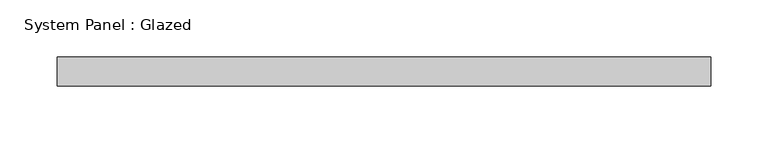
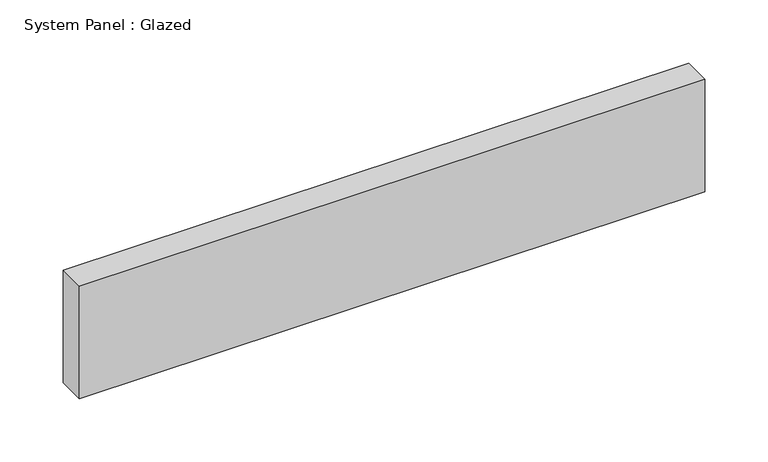
"""IFC4 building model written with IfcOpenShell, lengths in millimetres: plate geometry, System Panel : Glazed."""

from ifc_helpers import new_model, si_unit, origin, origin_with_axes, place, context, project, spatial, polyline, outline, extrude, source, transform, mapped, element, save


def system_panel_glazed_afc0885c(model_context):
    return source(origin(), model_context, "Body", "SweptSolid", [
        extrude(outline(polyline([(285.75, 19.05), (-285.75, 19.05), (-285.75, 44.45), (285.75, 44.45), (285.75, 19.05)])), origin_with_axes(), (0.0, 0.0, 1.0), 108.6326151),
    ])


if __name__ == "__main__":
    model = new_model("IFC4")
    model_context = context("Model", 3, world=origin())
    ifc_project = project(units=[si_unit("LENGTHUNIT", "METRE", prefix="MILLI")], contexts=[model_context])
    site = spatial("IfcSite", under=ifc_project)
    building = spatial("IfcBuilding", under=site)
    placement = place(None, origin())
    system_panel_glazed_shape = system_panel_glazed_afc0885c(model_context)
    element("IfcPlate", 1, ObjectType="System Panel : Glazed", at=placement, inside=building, context=model_context, shape_type="MappedRepresentation", body=[
        mapped(system_panel_glazed_shape, transform((0.0, 0.0, 0.0), x_axis=(1.0, 0.0, 0.0), y_axis=(0.0, 1.0, 0.0), z_axis=(0.0, 0.0, 1.0))),
    ])
    save(model, "model.ifc")

# Revit data of these elements
# Type "System Panel : Glazed"
#   Construction Type Id = "GSP4R"
#   Analytic Construction = "1/8 in Pilkington single glazing"
#   Visual Light Transmittance = 0.9
#   Solar Heat Gain Coefficient = 0.86
#   Heat Transfer Coefficient (U) = 1.18115 BTU/(h·ft²·°F)
#   Define Thermal Properties by = 1
# Element 1 (IfcPlate, "System Panel : Glazed")
#   Materials on its faces: "Glass"
# Materials
#   "Glass": class "Glass", colour RGB 0 128 192, transparency 0.75, Description = "Soda Lime Glass", Cost = 0
